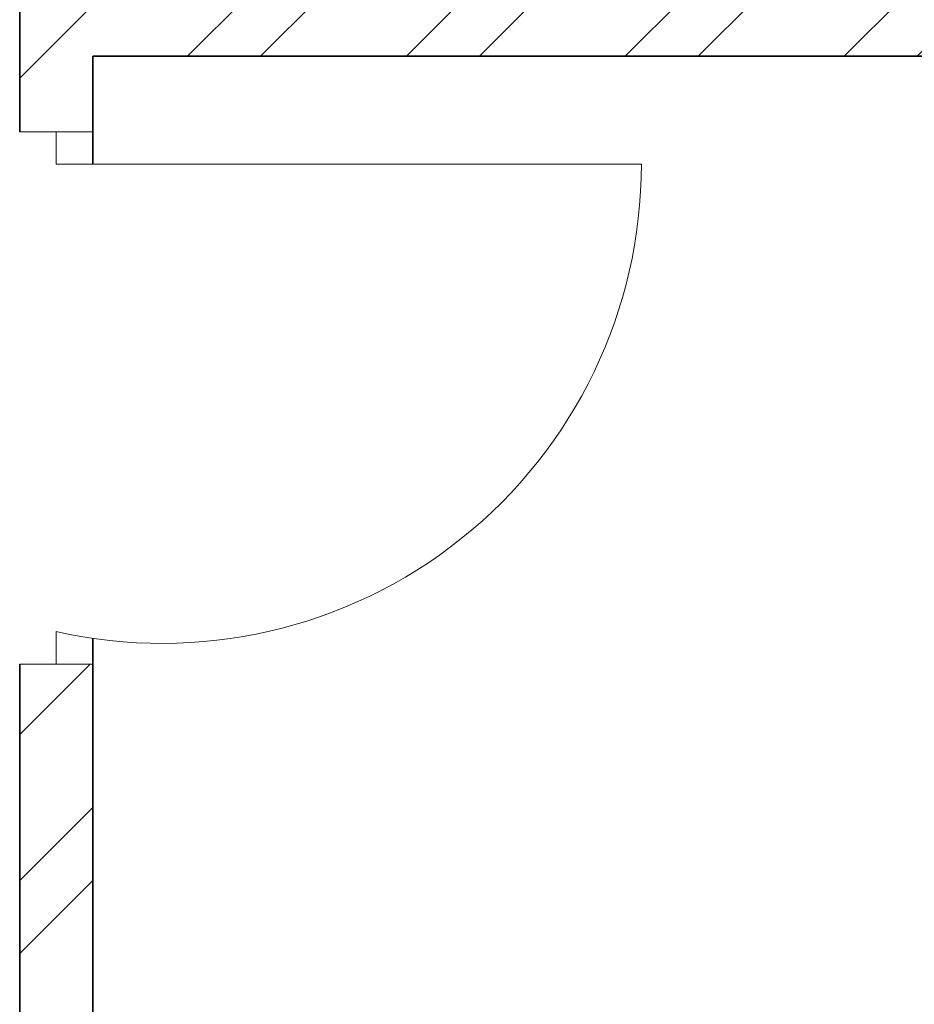
# Model space of a CAD drawing. Units: inches. Extents: x 2168 to 3056, y 1130 to 2629.
# Tile 12 of 42: x 2645 to 2700, y 2018 to 2079. Entities that reach past the tile are written whole.
import ezdxf

# ---------------------------------------------------------------- set-up
doc = ezdxf.new("R2010")
doc.units = ezdxf.units.IN
doc.layers.add('A-DOOR', color=21, linetype='Continuous', lineweight=18)
doc.layers.add('A-WALL', color=7, linetype='Continuous', lineweight=35)
doc.layers.add('A-WALL-PATT', color=143, linetype='Continuous', lineweight=13, true_color=0x7aafdf)

msp = doc.modelspace()

# ---------------------------------------------------------------- hatches: boundary and pattern name
at = {"layer": 'A-WALL-PATT'}
h = msp.add_hatch(dxfattribs=at)
h.set_pattern_fill('ANSI32', color=256)
h.paths.add_polyline_path([(2463.796, 2409.389), (2467.387, 2409.389), (2467.387, 2413.889), (2454.768, 2413.889), (2454.768, 2411.639), (2454.768, 2409.389), (2459.296, 2409.389), (2459.296, 2265.389), (2455.644, 2265.389), (2455.644, 2260.889), (2467.349, 2260.889), (2467.349, 2263.139), (2467.349, 2265.389), (2463.796, 2265.389)])
h.paths.add_polyline_path([(2431.596, 2413.889), (2409.647, 2413.889), (2409.647, 2409.389), (2431.596, 2409.389), (2431.596, 2411.639)])
h.paths.add_polyline_path([(2349.647, 2413.889), (2331.796, 2413.889), (2331.796, 2362.671), (2336.296, 2362.671), (2336.296, 2409.389), (2349.647, 2409.389), (2349.647, 2411.639)])
h.paths.add_polyline_path([(2634.149, 2411.639), (2634.149, 2413.889), (2562.293, 2413.889), (2562.293, 2409.389), (2595.796, 2409.389), (2595.796, 2280.309), (2595.826, 2280.309), (2595.826, 2265.389), (2499.91, 2265.389), (2499.91, 2260.889), (2550.796, 2260.889), (2550.796, 2117.308), (2555.296, 2117.308), (2555.296, 2168.08), (2571.93, 2168.08), (2571.93, 2176.889), (2559.796, 2176.889), (2559.796, 2256.389), (2640.796, 2256.389), (2640.796, 2176.889), (2626.428, 2176.889), (2626.428, 2168.08), (2645.296, 2168.08), (2645.296, 2116.637), (2649.796, 2116.637), (2649.796, 2260.889), (2691.251, 2260.889), (2691.251, 2263.139), (2691.251, 2265.389), (2670.655, 2265.389), (2670.655, 2265.365), (2600.296, 2265.365), (2600.296, 2280.258), (2600.296, 2409.389), (2634.149, 2409.389)])
h.paths.add_polyline_path([(2600.296, 2473.889), (2612.84, 2473.889), (2612.84, 2478.389), (2572.636, 2478.389), (2572.636, 2473.889), (2595.796, 2473.889), (2595.796, 2413.889), (2600.296, 2413.889)])
h.paths.add_polyline_path([(2535.796, 2473.889), (2548.636, 2473.889), (2548.636, 2478.389), (2531.396, 2478.389), (2531.396, 2413.889), (2521.6, 2413.889), (2521.6, 2409.389), (2539.239, 2409.389), (2539.239, 2411.639), (2539.239, 2413.889), (2535.796, 2413.889)])
h.paths.add_polyline_path([(2664.796, 2478.389), (2636.84, 2478.389), (2636.84, 2473.889), (2660.296, 2473.889), (2660.296, 2413.889), (2656.165, 2413.889), (2656.165, 2409.389), (2671.684, 2409.389), (2671.684, 2411.639), (2671.684, 2413.889), (2664.796, 2413.889)])
h.paths.add_polyline_path([(2705.942, 2413.889), (2695.684, 2413.889), (2695.684, 2409.389), (2705.942, 2409.389)])
h.paths.add_polyline_path([(2741.35, 2413.889), (2728.733, 2413.889), (2728.733, 2411.639), (2728.733, 2409.389), (2732.296, 2409.389), (2732.296, 2265.389), (2725.733, 2265.389), (2725.733, 2260.889), (2740.917, 2260.889), (2740.917, 2263.139), (2740.917, 2265.389), (2736.796, 2265.389), (2736.796, 2409.389), (2741.35, 2409.389)])
h.paths.add_polyline_path([(2785.655, 2413.889), (2764.546, 2413.889), (2764.486, 2409.389), (2785.655, 2409.389), (2785.655, 2411.639)])
h.paths.add_polyline_path([(2864.296, 2413.889), (2845.655, 2413.889), (2845.655, 2409.389), (2859.796, 2409.389), (2859.796, 2368.425), (2864.296, 2368.425)])
h.paths.add_polyline_path([(2864.296, 2308.425), (2862.046, 2308.425), (2859.796, 2308.425), (2859.796, 2265.389), (2774.483, 2265.389), (2774.483, 2263.139), (2774.483, 2260.889), (2781.796, 2260.889), (2781.796, 2226.654), (2786.296, 2226.654), (2786.296, 2260.889), (2859.796, 2260.889), (2859.796, 2241.352), (2864.296, 2241.352)])
h.paths.add_polyline_path([(2864.296, 2217.352), (2862.046, 2217.352), (2859.796, 2217.352), (2859.796, 2200.889), (2786.296, 2200.889), (2786.296, 2205.931), (2784.046, 2205.931), (2781.796, 2205.931), (2781.796, 2150.974), (2786.296, 2150.974), (2786.296, 2161.889), (2859.796, 2161.889), (2859.796, 2144.419), (2864.296, 2144.419)])
h.paths.add_polyline_path([(2859.796, 2196.389), (2859.796, 2166.389), (2786.296, 2166.389), (2786.296, 2196.389)], flags=16)
h.paths.add_polyline_path([(2864.296, 2108.419), (2862.046, 2108.419), (2859.796, 2108.419), (2859.796, 2080.889), (2786.296, 2080.889), (2786.296, 2111.993), (2781.796, 2111.993), (2781.796, 2080.889), (2649.796, 2080.889), (2649.796, 2086.036), (2647.546, 2086.036), (2645.296, 2086.036), (2645.296, 2071.739), (2649.796, 2071.739), (2649.796, 2076.389), (2781.796, 2076.389), (2781.796, 2041.792), (2786.296, 2041.792), (2786.296, 2076.389), (2859.796, 2076.389), (2859.796, 2058.577), (2864.296, 2058.577)])
h.paths.add_polyline_path([(2864.296, 2022.577), (2859.796, 2022.577), (2859.796, 1992.389), (2786.296, 1992.389), (2786.296, 1999.573), (2781.796, 1999.573), (2781.796, 1848.085), (2784.046, 1848.085), (2786.296, 1848.085), (2786.296, 1851.389), (2859.796, 1851.389), (2859.796, 1838.258), (2864.296, 1838.258)], flags=17)
h.paths.add_polyline_path([(2859.796, 1987.889), (2859.796, 1855.889), (2786.296, 1855.889), (2786.296, 1987.889)], flags=16)
h.paths.add_polyline_path([(2823.046, 1987.889), (2841.421, 1921.889), (2823.046, 1855.889)], flags=0)
h.paths.add_polyline_path([(2864.296, 1814.258), (2859.796, 1814.258), (2859.796, 1791.389), (2786.296, 1791.389), (2786.296, 1825.658), (2784.046, 1825.658), (2781.796, 1825.658), (2781.796, 1791.389), (2720.155, 1791.389), (2720.155, 1791.265), (2649.796, 1791.265), (2649.796, 1806.159), (2649.796, 2038.983), (2647.546, 2038.983), (2645.296, 2038.983), (2645.296, 1783.925), (2649.796, 1783.925), (2649.796, 1786.889), (2781.796, 1786.889), (2781.796, 1746.789), (2786.296, 1746.789), (2786.296, 1786.889), (2859.796, 1786.889), (2859.796, 1770.083), (2864.296, 1770.083)])
h.paths.add_polyline_path([(2864.296, 1734.083), (2862.046, 1734.083), (2859.796, 1734.083), (2859.796, 1705.889), (2786.296, 1705.889), (2786.296, 1714.166), (2781.796, 1714.166), (2781.796, 1660.527), (2786.296, 1660.527), (2786.296, 1666.889), (2859.796, 1666.889), (2859.796, 1648.342), (2864.296, 1648.342)])
h.paths.add_polyline_path([(2786.296, 1701.389), (2859.796, 1701.389), (2859.796, 1671.389), (2786.296, 1671.389)], flags=16)
h.paths.add_polyline_path([(2649.796, 1756.576), (2647.546, 1756.576), (2645.296, 1756.576), (2645.296, 1606.889), (2555.296, 1606.889), (2555.296, 1749.513), (2553.046, 1749.513), (2550.796, 1749.513), (2550.796, 1606.889), (2503.006, 1606.889), (2503.006, 1604.639), (2503.006, 1602.389), (2595.796, 1602.389), (2595.849, 1602.389), (2595.849, 1587.495), (2595.796, 1458.389), (2561.502, 1458.389), (2561.502, 1456.139), (2561.502, 1453.889), (2595.796, 1453.889), (2595.796, 1381.889), (2573.438, 1381.889), (2573.438, 1377.389), (2613.01, 1377.389), (2613.01, 1379.639), (2613.01, 1381.889), (2600.296, 1381.889), (2600.296, 1453.889), (2634.327, 1453.889), (2634.327, 1458.389), (2600.296, 1458.389), (2600.296, 1602.389), (2670.655, 1602.389), (2694.095, 1602.389), (2694.095, 1606.889), (2649.796, 1606.889)])
h.paths.add_polyline_path([(2736.796, 1602.389), (2741.562, 1602.389), (2741.562, 1606.889), (2726.203, 1606.889), (2726.203, 1604.639), (2726.203, 1602.389), (2732.296, 1602.389), (2732.296, 1458.389), (2727.899, 1458.389), (2727.899, 1453.889), (2740.821, 1453.889), (2740.821, 1456.139), (2740.821, 1458.389), (2736.796, 1458.389)])
h.paths.add_polyline_path([(2859.796, 1606.889), (2786.296, 1606.889), (2786.296, 1637.334), (2784.046, 1637.334), (2781.796, 1637.334), (2781.796, 1606.889), (2775.612, 1606.889), (2775.612, 1602.389), (2859.796, 1602.389)])
h.paths.add_polyline_path([(2864.296, 1624.342), (2862.046, 1624.342), (2859.796, 1624.342), (2859.796, 1570.39), (2864.296, 1570.39)])
h.paths.add_polyline_path([(2864.296, 1510.39), (2862.046, 1510.39), (2859.796, 1510.39), (2859.796, 1458.389), (2846.735, 1458.389), (2846.735, 1456.139), (2846.735, 1453.889), (2864.296, 1453.889)])
h.paths.add_polyline_path([(2786.735, 1458.389), (2765.444, 1458.389), (2765.444, 1453.889), (2786.735, 1453.889)])
h.paths.add_polyline_path([(2706.004, 1458.389), (2695.36, 1458.389), (2695.36, 1453.889), (2706.004, 1453.889), (2706.004, 1456.139)])
h.paths.add_polyline_path([(2671.36, 1456.139), (2671.36, 1458.389), (2655.986, 1458.389), (2655.986, 1456.139), (2655.986, 1453.889), (2660.296, 1453.889), (2660.296, 1381.889), (2637.01, 1381.889), (2637.01, 1377.389), (2664.796, 1377.389), (2664.796, 1453.889), (2671.36, 1453.889)], flags=17)
h.paths.add_polyline_path([(2539.829, 1458.389), (2520.237, 1458.389), (2520.237, 1453.889), (2531.296, 1453.889), (2531.296, 1377.389), (2546.449, 1377.389), (2546.449, 1379.639), (2546.449, 1381.889), (2535.796, 1381.889), (2535.796, 1453.889), (2539.829, 1453.889)], flags=17)
h.paths.add_polyline_path([(2496.237, 1458.389), (2489.13, 1458.389), (2489.13, 1453.889), (2496.237, 1453.889), (2496.237, 1456.139)])
h.paths.add_polyline_path([(2467.433, 1456.139), (2467.433, 1458.389), (2463.796, 1458.389), (2463.796, 1602.389), (2468.242, 1602.389), (2468.242, 1605.7), (2468.242, 1606.889), (2454.602, 1606.889), (2454.602, 1602.389), (2459.296, 1602.389), (2459.296, 1458.389), (2454.24, 1458.389), (2454.24, 1453.889), (2467.433, 1453.889)])
h.paths.add_polyline_path([(2431.601, 1456.139), (2431.601, 1458.389), (2411.386, 1458.389), (2411.386, 1453.889), (2431.601, 1453.889)])
h.paths.add_polyline_path([(2351.386, 1458.389), (2336.296, 1458.389), (2336.296, 1490.693), (2334.046, 1490.693), (2331.796, 1490.693), (2331.796, 1453.889), (2351.386, 1453.889), (2351.386, 1456.139)])
h.paths.add_polyline_path([(2336.296, 1629.705), (2331.796, 1629.705), (2331.796, 1552.317), (2336.296, 1552.317), (2336.296, 1602.389), (2406.655, 1602.389), (2423.472, 1602.389), (2423.472, 1606.889), (2418.796, 1606.889), (2418.796, 1643.678), (2416.546, 1643.678), (2414.296, 1643.678), (2414.296, 1606.889), (2336.296, 1606.889)])
h.paths.add_polyline_path([(2418.796, 1714.384), (2414.296, 1714.384), (2414.296, 1705.889), (2336.296, 1705.889), (2336.296, 1731.324), (2334.046, 1731.324), (2331.796, 1731.324), (2331.796, 1653.705), (2334.046, 1653.705), (2336.296, 1653.705), (2336.296, 1666.889), (2414.296, 1666.889), (2414.296, 1663.589), (2418.796, 1663.589)])
h.paths.add_polyline_path([(2336.296, 1701.389), (2414.296, 1701.389), (2414.296, 1671.389), (2336.296, 1671.389)], flags=16)
h.paths.add_polyline_path([(2555.296, 2040.059), (2550.796, 2040.059), (2550.796, 1791.389), (2550.561, 1791.205), (2480.202, 1791.205), (2418.796, 1791.389), (2418.796, 1825.448), (2416.546, 1825.448), (2414.296, 1825.448), (2414.296, 1791.389), (2336.296, 1791.389), (2336.296, 1806.409), (2331.796, 1806.409), (2331.796, 1767.324), (2336.296, 1767.324), (2336.296, 1786.889), (2414.296, 1786.889), (2414.296, 1745.457), (2418.796, 1745.457), (2418.796, 1786.889), (2550.796, 1786.889), (2550.796, 1783.011), (2555.296, 1783.011)])
h.paths.add_polyline_path([(2418.796, 1923.389), (2423.207, 1923.389), (2423.207, 1925.639), (2423.207, 1927.889), (2418.796, 1927.889), (2418.796, 2000.048), (2414.296, 2000.048), (2414.296, 1992.389), (2336.296, 1992.389), (2336.296, 1987.889), (2414.296, 1987.889), (2414.296, 1855.889), (2336.296, 1855.889), (2336.296, 1851.389), (2414.296, 1851.389), (2414.296, 1846.759), (2418.796, 1846.759)], flags=17)
h.paths.add_polyline_path([(2336.296, 2019.294), (2334.046, 2019.294), (2331.796, 2019.294), (2331.796, 1830.409), (2336.296, 1830.409)], flags=17)
h.paths.add_polyline_path([(2550.796, 1927.889), (2453.541, 1927.889), (2453.541, 1925.639), (2453.541, 1923.389), (2550.796, 1923.389)], flags=17)
h.paths.add_polyline_path([(2744.987, 1927.889), (2649.796, 1927.889), (2649.796, 1923.389), (2744.987, 1923.389), (2744.987, 1925.639)], flags=17)
h.paths.add_polyline_path([(2555.296, 2086.458), (2553.046, 2086.458), (2550.796, 2086.458), (2550.796, 2080.889), (2418.796, 2080.889), (2336.296, 2080.889), (2336.296, 2115.399), (2334.046, 2115.399), (2331.796, 2115.399), (2331.796, 2055.294), (2336.296, 2055.294), (2336.296, 2076.389), (2550.796, 2076.389), (2550.796, 2071.538), (2555.296, 2071.538)])
h.paths.add_polyline_path([(2418.796, 2121.389), (2414.296, 2121.389), (2414.296, 2080.889), (2418.796, 2080.889)])
h.paths.add_polyline_path([(2418.796, 2076.389), (2414.296, 2076.389), (2414.296, 2035.123), (2418.796, 2035.123)])
h.paths.add_polyline_path([(2422.868, 2263.139), (2422.868, 2265.389), (2406.655, 2265.389), (2406.655, 2265.359), (2336.296, 2265.359), (2336.296, 2280.252), (2336.296, 2302.671), (2334.046, 2302.671), (2331.796, 2302.671), (2331.796, 2246.853), (2336.296, 2246.853), (2336.296, 2260.889), (2414.296, 2260.889), (2414.296, 2223.996), (2418.796, 2223.996), (2418.796, 2260.889), (2422.868, 2260.889)])
h.paths.add_polyline_path([(2418.796, 2204.783), (2416.546, 2204.783), (2414.296, 2204.783), (2414.296, 2200.889), (2336.296, 2200.889), (2336.296, 2220.853), (2331.796, 2220.853), (2331.796, 2151.399), (2336.296, 2151.399), (2336.296, 2161.889), (2414.296, 2161.889), (2414.296, 2153.726), (2418.796, 2153.726)])
h.paths.add_polyline_path([(2414.296, 2196.389), (2414.296, 2166.389), (2336.296, 2166.389), (2336.296, 2196.389)], flags=16)
h.paths.add_polyline_path([(2375.296, 2181.389), (2336.296, 2166.389), (2336.296, 2196.389)], flags=0)
h.paths.add_polyline_path([(2809.595, 2172.34), (2838.804, 2172.34), (2838.804, 2190.997), (2809.595, 2190.997)], flags=8)
h.paths.add_polyline_path([(2849.75, 1919.585), (2849.75, 1952.672), (2831.093, 1952.672), (2831.093, 1919.585)], flags=8)
h.paths.add_polyline_path([(2808.875, 1901.967), (2808.875, 1937.85), (2790.149, 1937.85), (2790.149, 1901.967)], flags=8)
h.paths.add_polyline_path([(2806.285, 1671.896), (2835.493, 1671.896), (2835.493, 1690.553), (2806.285, 1690.553)], flags=8)
h.paths.add_polyline_path([(2353.186, 1676.549), (2382.395, 1676.549), (2382.395, 1695.207), (2353.186, 1695.207)], flags=8)
h.paths.add_polyline_path([(2360.083, 1832.308), (2389.241, 1832.308), (2389.241, 1850.966), (2360.083, 1850.966)], flags=25)
h.paths.add_polyline_path([(2354.822, 2167.823), (2384.031, 2167.823), (2384.031, 2186.481), (2354.822, 2186.481)], flags=8)

# ---------------------------------------------------------------- linework, layer by layer
at = {"layer": 'A-DOOR'}
for p, q in [((2645.296, 2071.739), (2649.796, 2071.739)), ((2649.796, 2071.739), (2647.546, 2071.739)), ((2647.546, 2071.739), (2647.546, 2069.739)), ((2647.546, 2069.739), (2683.546, 2069.739)), ((2647.546, 2038.983), (2647.546, 2040.983)), ((2645.296, 2038.983), (2649.796, 2038.983)), ((2649.796, 2038.983), (2647.546, 2038.983))]:
    msp.add_line(p, q, dxfattribs=at)
msp.add_arc((2654.061, 2069.739), 29.484, 257.233, 0, dxfattribs=at)
at = {"layer": 'A-WALL'}
for p, q in [((2645.296, 2086.036), (2645.296, 2071.739)), ((2649.796, 2076.389), (2781.796, 2076.389)), ((2649.796, 2069.739), (2649.796, 2076.389)), ((2649.796, 1791.389), (2649.796, 2040.564)), ((2645.296, 2038.983), (2645.296, 1783.925))]:
    msp.add_line(p, q, dxfattribs=at)

doc.saveas('drawing.dxf')
